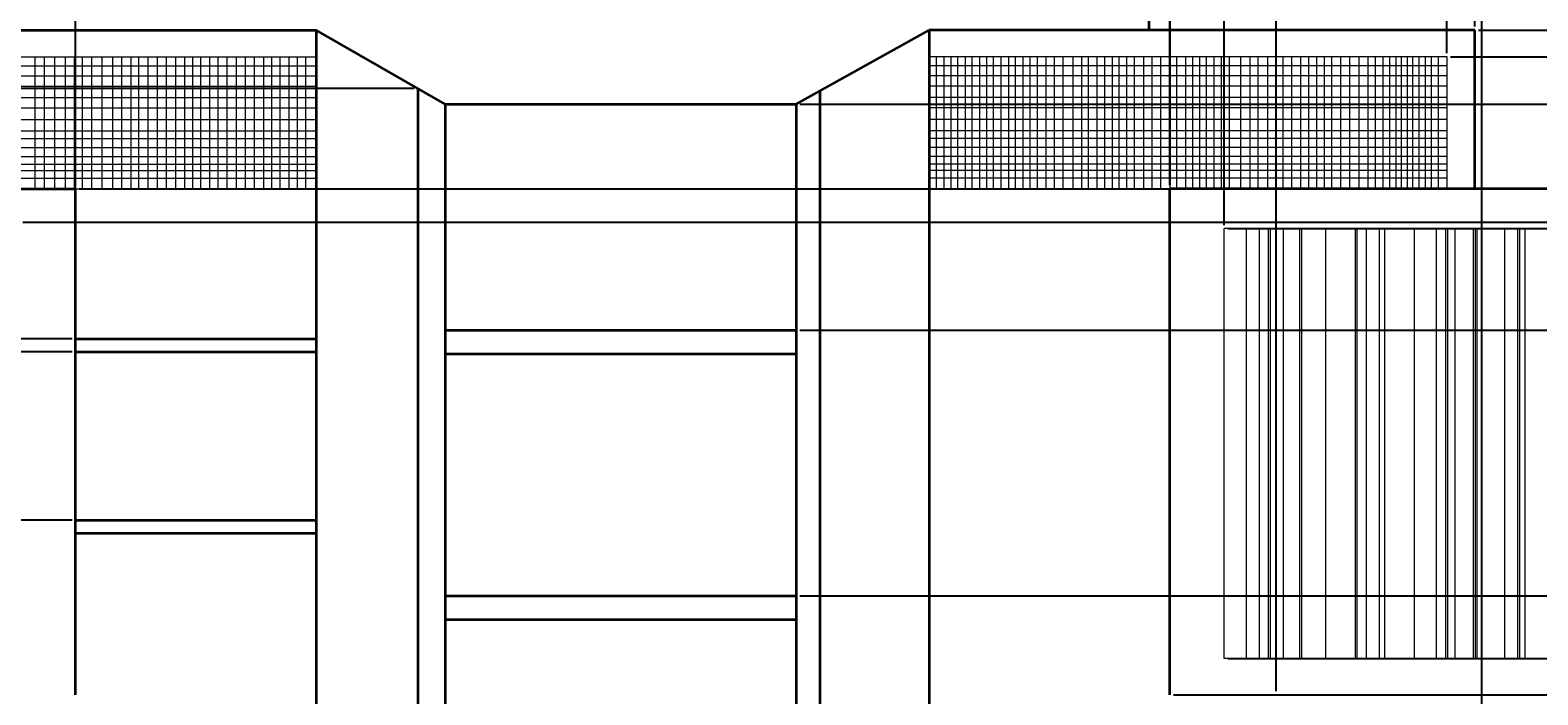
# Model space of a CAD drawing. Units: inches. Extents: x -10 to 130, y -32 to 34.
# Tile 16 of 22: x 49 to 75, y 6 to 18. Entities that reach past the tile are written whole.
import ezdxf

# ---------------------------------------------------------------- set-up
doc = ezdxf.new("R2010")
doc.units = ezdxf.units.IN
doc.header["$MEASUREMENT"] = 0
for name, color, linetype, lineweight in [('A-ANNO-DIMS', 2, 'Continuous', 18), ('A-ELEV', 7, 'Continuous', 35), ('A-GLAZ', 4, 'Continuous', 18)]:
    doc.layers.add(name, color=color, linetype=linetype, lineweight=lineweight)
doc.styles.get("Standard").update_dxf_attribs({"font": 'arial.ttf'})
doc.dimstyles.get("Standard").update_dxf_attribs({"dimtxt": 0.18, "dimasz": 0.18, "dimexe": 0.18, "dimexo": 0.0625, "dimgap": 0.09, "dimtad": 0, "dimtih": 1, "dimtoh": 1, "dimdec": 4, "dimzin": 0, "dimdsep": 46, "dimtxsty": 'Standard', "dimcen": 0.09, "dimadec": 0, "dimazin": 0, "dimtfac": 1, "dimtdec": 4, "dimtofl": 0, "dimtmove": 0, "dimatfit": 3, "dimfxl": 1, "dimtolj": 1, "dimtzin": 0, "dimarcsym": 0})

# ---------------------------------------------------------------- blocks, each defined once
blk = doc.blocks.new('*D2')
at = {"layer": 'A-ANNO-DIMS', "color": 0, "lineweight": -2, "transparency": 16777216}
for p, q in [((68.738, 27.199), (129.508, 27.199)), ((129.328, 27.019), (129.328, 3.074)), ((129.328, -21.234), (129.328, 2.71)), ((107.996, -21.414), (129.508, -21.414))]:
    blk.add_line(p, q, dxfattribs=at)
at = {"layer": 'A-ANNO-DIMS', "color": 0, "transparency": 16777216}
for points in [[(129.298, 27.019), (129.358, 27.019), (129.328, 27.199)], [(129.298, -21.234), (129.358, -21.234), (129.328, -21.414)]]:
    blk.add_solid(points, dxfattribs=at)
at = {"layer": 'Defpoints', "color": 0, "transparency": 16777216}
for p in [(68.676, 27.199), (129.328, 27.199), (107.933, -21.414)]:
    blk.add_point(p, dxfattribs=at)
at = {"layer": 'A-ANNO-DIMS', "color": 0, "transparency": 16777216, "insert": (129.328, 2.892), "char_height": 0.18, "attachment_point": 5}
blk.add_mtext('\\A1;48.61', dxfattribs=at)
blk = doc.blocks.new('*D7')
at = {"layer": 'A-ANNO-DIMS', "color": 0, "lineweight": -2, "transparency": 16777216}
for p, q in [((42.614, 6.07), (42.614, 33.879)), ((42.794, 33.699), (45.888, 33.699)), ((49.766, 33.699), (46.672, 33.699)), ((49.946, 6.07), (49.946, 33.879))]:
    blk.add_line(p, q, dxfattribs=at)
at = {"layer": 'A-ANNO-DIMS', "color": 0, "transparency": 16777216}
for points in [[(42.794, 33.729), (42.794, 33.669), (42.614, 33.699)], [(49.766, 33.729), (49.766, 33.669), (49.946, 33.699)]]:
    blk.add_solid(points, dxfattribs=at)
at = {"layer": 'Defpoints', "color": 0, "transparency": 16777216}
for p in [(49.946, 33.699), (42.614, 6.007), (49.946, 6.007)]:
    blk.add_point(p, dxfattribs=at)
at = {"layer": 'A-ANNO-DIMS', "color": 0, "transparency": 16777216, "insert": (46.28, 33.699), "char_height": 0.18, "attachment_point": 5}
blk.add_mtext('\\A1;7.332', dxfattribs=at)
blk = doc.blocks.new('*D8')
at = {"layer": 'A-ANNO-DIMS', "color": 0, "lineweight": -2, "transparency": 16777216}
for p, q in [((68.676, 17.67), (68.676, 33.879)), ((68.856, 33.699), (69.393, 33.699)), ((70.718, 33.699), (70.181, 33.699)), ((70.898, 6.07), (70.898, 33.879))]:
    blk.add_line(p, q, dxfattribs=at)
at = {"layer": 'A-ANNO-DIMS', "color": 0, "transparency": 16777216}
for points in [[(68.856, 33.729), (68.856, 33.669), (68.676, 33.699)], [(70.718, 33.729), (70.718, 33.669), (70.898, 33.699)]]:
    blk.add_solid(points, dxfattribs=at)
at = {"layer": 'Defpoints', "color": 0, "transparency": 16777216}
for p in [(70.898, 33.699), (68.676, 17.607), (70.898, 6.007)]:
    blk.add_point(p, dxfattribs=at)
at = {"layer": 'A-ANNO-DIMS', "color": 0, "transparency": 16777216, "insert": (69.787, 33.699), "char_height": 0.18, "attachment_point": 5}
blk.add_mtext('\\A1;2.222', dxfattribs=at)
blk = doc.blocks.new('*D9')
at = {"layer": 'A-ANNO-DIMS', "color": 0, "lineweight": -2, "transparency": 16777216}
for p, q in [((70.898, 6.07), (70.898, 33.879)), ((71.078, 33.699), (75.697, 33.699)), ((81.225, 33.699), (76.607, 33.699)), ((81.405, 6.07), (81.405, 33.879))]:
    blk.add_line(p, q, dxfattribs=at)
at = {"layer": 'A-ANNO-DIMS', "color": 0, "transparency": 16777216}
for points in [[(71.078, 33.729), (71.078, 33.669), (70.898, 33.699)], [(81.225, 33.729), (81.225, 33.669), (81.405, 33.699)]]:
    blk.add_solid(points, dxfattribs=at)
at = {"layer": 'Defpoints', "color": 0, "transparency": 16777216}
for p in [(81.405, 33.699), (70.898, 6.007), (81.405, 6.007)]:
    blk.add_point(p, dxfattribs=at)
at = {"layer": 'A-ANNO-DIMS', "color": 0, "transparency": 16777216, "insert": (76.152, 33.699), "char_height": 0.18, "attachment_point": 5}
blk.add_mtext('\\A1;10.507', dxfattribs=at)
blk = doc.blocks.new('*D28')
at = {"layer": 'A-ANNO-DIMS', "color": 0, "lineweight": -2, "transparency": 16777216}
for p, q in [((21.715, 14.903), (21.715, 33.879)), ((21.895, 33.699), (35.436, 33.699)), ((49.766, 33.699), (36.226, 33.699)), ((49.946, 14.903), (49.946, 33.879))]:
    blk.add_line(p, q, dxfattribs=at)
at = {"layer": 'A-ANNO-DIMS', "color": 0, "transparency": 16777216}
for points in [[(21.895, 33.729), (21.895, 33.669), (21.715, 33.699)], [(49.766, 33.729), (49.766, 33.669), (49.946, 33.699)]]:
    blk.add_solid(points, dxfattribs=at)
at = {"layer": 'Defpoints', "color": 0, "transparency": 16777216}
for p in [(49.946, 33.699), (21.715, 14.841), (49.946, 14.841)]:
    blk.add_point(p, dxfattribs=at)
at = {"layer": 'A-ANNO-DIMS', "color": 0, "transparency": 16777216, "insert": (35.831, 33.699), "char_height": 0.18, "attachment_point": 5}
blk.add_mtext('\\A1;28.23', dxfattribs=at)
blk = doc.blocks.new('*D29')
at = {"layer": 'A-ANNO-DIMS', "color": 0, "lineweight": -2, "transparency": 16777216}
for p, q in [((69.045, 14.903), (69.045, 33.879)), ((69.225, 33.699), (82.743, 33.699)), ((97.053, 33.699), (83.534, 33.699)), ((97.233, 14.903), (97.233, 33.879))]:
    blk.add_line(p, q, dxfattribs=at)
at = {"layer": 'A-ANNO-DIMS', "color": 0, "transparency": 16777216}
for points in [[(69.225, 33.729), (69.225, 33.669), (69.045, 33.699)], [(97.053, 33.729), (97.053, 33.669), (97.233, 33.699)]]:
    blk.add_solid(points, dxfattribs=at)
at = {"layer": 'Defpoints', "color": 0, "transparency": 16777216}
for p in [(97.233, 33.699), (69.045, 14.841), (97.233, 14.841)]:
    blk.add_point(p, dxfattribs=at)
at = {"layer": 'A-ANNO-DIMS', "color": 0, "transparency": 16777216, "insert": (83.139, 33.699), "char_height": 0.18, "attachment_point": 5}
blk.add_mtext('\\A1;28.19', dxfattribs=at)
blk = doc.blocks.new('*D34')
at = {"layer": 'A-ANNO-DIMS', "color": 0, "lineweight": -2, "transparency": 16777216}
for p, q in [((13.34, 6.007), (-9.564, 6.007)), ((-9.384, 5.827), (-9.384, 3.941)), ((-9.384, 1.691), (-9.384, 3.577)), ((70.835, 1.511), (-9.564, 1.511))]:
    blk.add_line(p, q, dxfattribs=at)
at = {"layer": 'A-ANNO-DIMS', "color": 0, "transparency": 16777216}
for points in [[(-9.414, 5.827), (-9.354, 5.827), (-9.384, 6.007)], [(-9.414, 1.691), (-9.354, 1.691), (-9.384, 1.511)]]:
    blk.add_solid(points, dxfattribs=at)
at = {"layer": 'Defpoints', "color": 0, "transparency": 16777216}
for p in [(-9.384, 6.007), (13.402, 6.007), (70.898, 1.511)]:
    blk.add_point(p, dxfattribs=at)
at = {"layer": 'A-ANNO-DIMS', "color": 0, "transparency": 16777216, "insert": (-9.384, 3.759), "char_height": 0.18, "attachment_point": 5}
blk.add_mtext('\\A1;4.497', dxfattribs=at)
blk = doc.blocks.new('*D48')
at = {"layer": 'A-ANNO-DIMS', "color": 0, "lineweight": -2, "transparency": 16777216}
for p, q in [((44.76, -13.293), (44.76, 33.879)), ((44.94, 33.699), (59.231, 33.699)), ((74.312, 33.699), (60.021, 33.699)), ((74.492, -13.293), (74.492, 33.879))]:
    blk.add_line(p, q, dxfattribs=at)
at = {"layer": 'A-ANNO-DIMS', "color": 0, "transparency": 16777216}
for points in [[(44.94, 33.729), (44.94, 33.669), (44.76, 33.699)], [(74.312, 33.729), (74.312, 33.669), (74.492, 33.699)]]:
    blk.add_solid(points, dxfattribs=at)
at = {"layer": 'Defpoints', "color": 0, "transparency": 16777216}
for p in [(74.492, 33.699), (44.76, -13.356), (74.492, -13.356)]:
    blk.add_point(p, dxfattribs=at)
at = {"layer": 'A-ANNO-DIMS', "color": 0, "transparency": 16777216, "insert": (59.626, 33.699), "char_height": 0.18, "attachment_point": 5}
blk.add_mtext('\\A1;29.73', dxfattribs=at)
blk = doc.blocks.new('*D60')
at = {"layer": 'A-ANNO-DIMS', "color": 0, "lineweight": -2, "transparency": 16777216}
for p, q in [((74.492, -13.293), (74.492, 33.879)), ((74.672, 33.699), (78.041, 33.699)), ((82.197, 33.699), (78.828, 33.699)), ((82.377, -15.202), (82.377, 33.879))]:
    blk.add_line(p, q, dxfattribs=at)
at = {"layer": 'A-ANNO-DIMS', "color": 0, "transparency": 16777216}
for points in [[(74.672, 33.729), (74.672, 33.669), (74.492, 33.699)], [(82.197, 33.729), (82.197, 33.669), (82.377, 33.699)]]:
    blk.add_solid(points, dxfattribs=at)
at = {"layer": 'Defpoints', "color": 0, "transparency": 16777216}
for p in [(82.377, 33.699), (74.492, -13.356), (82.377, -15.264)]:
    blk.add_point(p, dxfattribs=at)
at = {"layer": 'A-ANNO-DIMS', "color": 0, "transparency": 16777216, "insert": (78.435, 33.699), "char_height": 0.18, "attachment_point": 5}
blk.add_mtext('\\A1;7.885', dxfattribs=at)
blk = doc.blocks.new('*D72')
at = {"layer": 'A-ANNO-DIMS', "color": 0, "lineweight": -2, "transparency": 16777216}
for p, q in [((55.918, 16.529), (55.918, -28.129)), ((62.934, 16.482), (62.934, -28.129)), ((56.098, -27.949), (59.033, -27.949)), ((62.754, -27.949), (59.819, -27.949))]:
    blk.add_line(p, q, dxfattribs=at)
at = {"layer": 'A-ANNO-DIMS', "color": 0, "transparency": 16777216}
for points in [[(56.098, -27.919), (56.098, -27.979), (55.918, -27.949)], [(62.754, -27.919), (62.754, -27.979), (62.934, -27.949)]]:
    blk.add_solid(points, dxfattribs=at)
at = {"layer": 'Defpoints', "color": 0, "transparency": 16777216}
for p in [(55.918, 16.591), (62.934, 16.545), (62.934, -27.949)]:
    blk.add_point(p, dxfattribs=at)
at = {"layer": 'A-ANNO-DIMS', "color": 0, "transparency": 16777216, "insert": (59.426, -27.949), "char_height": 0.18, "attachment_point": 5}
blk.add_mtext('\\A1;7.016', dxfattribs=at)
blk = doc.blocks.new('*D73')
at = {"layer": 'A-ANNO-DIMS', "color": 0, "lineweight": -2, "transparency": 16777216}
for p, q in [((56.395, 16.255), (56.395, -28.129)), ((62.526, 16.255), (62.526, -28.129)), ((56.575, -27.949), (59.083, -27.949)), ((62.346, -27.949), (59.837, -27.949))]:
    blk.add_line(p, q, dxfattribs=at)
at = {"layer": 'A-ANNO-DIMS', "color": 0, "transparency": 16777216}
for points in [[(56.575, -27.919), (56.575, -27.979), (56.395, -27.949)], [(62.346, -27.919), (62.346, -27.979), (62.526, -27.949)]]:
    blk.add_solid(points, dxfattribs=at)
at = {"layer": 'Defpoints', "color": 0, "transparency": 16777216}
for p in [(56.395, 16.317), (62.526, 16.317), (62.526, -27.949)]:
    blk.add_point(p, dxfattribs=at)
at = {"layer": 'A-ANNO-DIMS', "color": 0, "transparency": 16777216, "insert": (59.46, -27.949), "char_height": 0.18, "attachment_point": 5}
blk.add_mtext('\\A1;6.131', dxfattribs=at)
blk = doc.blocks.new('*D74')
at = {"layer": 'A-ANNO-DIMS', "color": 0, "lineweight": -2, "transparency": 16777216}
for p, q in [((54.085, 17.607), (-9.564, 17.607)), ((-9.384, 17.427), (-9.384, 17.281)), ((-9.384, 16.771), (-9.384, 16.917)), ((55.856, 16.591), (-9.564, 16.591))]:
    blk.add_line(p, q, dxfattribs=at)
at = {"layer": 'A-ANNO-DIMS', "color": 0, "transparency": 16777216}
for points in [[(-9.414, 17.427), (-9.354, 17.427), (-9.384, 17.607)], [(-9.414, 16.771), (-9.354, 16.771), (-9.384, 16.591)]]:
    blk.add_solid(points, dxfattribs=at)
at = {"layer": 'Defpoints', "color": 0, "transparency": 16777216}
for p in [(54.147, 17.607), (-9.384, 16.591), (55.918, 16.591)]:
    blk.add_point(p, dxfattribs=at)
at = {"layer": 'A-ANNO-DIMS', "color": 0, "transparency": 16777216, "insert": (-9.384, 17.099), "char_height": 0.18, "attachment_point": 5}
blk.add_mtext('\\A1;1.02', dxfattribs=at)
blk = doc.blocks.new('*D79')
at = {"layer": 'A-ANNO-DIMS', "color": 0, "lineweight": -2, "transparency": 16777216}
for p, q in [((62.588, 7.736), (129.508, 7.736)), ((129.328, 7.556), (129.328, 5.559)), ((129.328, 3.198), (129.328, 5.195)), ((62.588, 3.018), (129.508, 3.018))]:
    blk.add_line(p, q, dxfattribs=at)
at = {"layer": 'A-ANNO-DIMS', "color": 0, "transparency": 16777216}
for points in [[(129.298, 7.556), (129.358, 7.556), (129.328, 7.736)], [(129.298, 3.198), (129.358, 3.198), (129.328, 3.018)]]:
    blk.add_solid(points, dxfattribs=at)
at = {"layer": 'Defpoints', "color": 0, "transparency": 16777216}
for p in [(62.526, 7.736), (129.328, 7.736), (62.526, 3.018)]:
    blk.add_point(p, dxfattribs=at)
at = {"layer": 'A-ANNO-DIMS', "color": 0, "transparency": 16777216, "insert": (129.328, 5.377), "char_height": 0.18, "attachment_point": 5}
blk.add_mtext('\\A1;4.718', dxfattribs=at)
blk = doc.blocks.new('*D80')
at = {"layer": 'A-ANNO-DIMS', "color": 0, "lineweight": -2, "transparency": 16777216}
for p, q in [((62.588, 12.373), (129.508, 12.373)), ((129.328, 12.193), (129.328, 10.237)), ((129.328, 7.916), (129.328, 9.873)), ((62.588, 7.736), (129.508, 7.736))]:
    blk.add_line(p, q, dxfattribs=at)
at = {"layer": 'A-ANNO-DIMS', "color": 0, "transparency": 16777216}
for points in [[(129.298, 12.193), (129.358, 12.193), (129.328, 12.373)], [(129.298, 7.916), (129.358, 7.916), (129.328, 7.736)]]:
    blk.add_solid(points, dxfattribs=at)
at = {"layer": 'Defpoints', "color": 0, "transparency": 16777216}
for p in [(62.526, 12.373), (129.328, 12.373), (62.526, 7.736)]:
    blk.add_point(p, dxfattribs=at)
at = {"layer": 'A-ANNO-DIMS', "color": 0, "transparency": 16777216, "insert": (129.328, 10.055), "char_height": 0.18, "attachment_point": 5}
blk.add_mtext('\\A1;4.64', dxfattribs=at)
blk = doc.blocks.new('*D81')
at = {"layer": 'A-ANNO-DIMS', "color": 0, "lineweight": -2, "transparency": 16777216}
for p, q in [((62.588, 16.317), (129.508, 16.317)), ((129.328, 16.137), (129.328, 14.527)), ((129.328, 12.553), (129.328, 14.163)), ((62.588, 12.373), (129.508, 12.373))]:
    blk.add_line(p, q, dxfattribs=at)
at = {"layer": 'A-ANNO-DIMS', "color": 0, "transparency": 16777216}
for points in [[(129.298, 16.137), (129.358, 16.137), (129.328, 16.317)], [(129.298, 12.553), (129.358, 12.553), (129.328, 12.373)]]:
    blk.add_solid(points, dxfattribs=at)
at = {"layer": 'Defpoints', "color": 0, "transparency": 16777216}
for p in [(62.526, 16.317), (129.328, 16.317), (62.526, 12.373)]:
    blk.add_point(p, dxfattribs=at)
at = {"layer": 'A-ANNO-DIMS', "color": 0, "transparency": 16777216, "insert": (129.328, 14.345), "char_height": 0.18, "attachment_point": 5}
blk.add_mtext('\\A1;3.94', dxfattribs=at)
blk = doc.blocks.new('*D87')
at = {"layer": 'A-ANNO-DIMS', "color": 0, "lineweight": -2, "transparency": 16777216}
for p, q in [((49.884, 14.841), (-9.564, 14.841)), ((-9.384, 14.661), (-9.384, 13.713)), ((-9.384, 12.402), (-9.384, 13.35)), ((49.884, 12.222), (-9.564, 12.222))]:
    blk.add_line(p, q, dxfattribs=at)
at = {"layer": 'A-ANNO-DIMS', "color": 0, "transparency": 16777216}
for points in [[(-9.414, 14.661), (-9.354, 14.661), (-9.384, 14.841)], [(-9.414, 12.402), (-9.354, 12.402), (-9.384, 12.222)]]:
    blk.add_solid(points, dxfattribs=at)
at = {"layer": 'Defpoints', "color": 0, "transparency": 16777216}
for p in [(49.946, 14.841), (-9.384, 12.222), (49.946, 12.222)]:
    blk.add_point(p, dxfattribs=at)
at = {"layer": 'A-ANNO-DIMS', "color": 0, "transparency": 16777216, "insert": (-9.384, 13.532), "char_height": 0.18, "attachment_point": 5}
blk.add_mtext('\\A1;2.619', dxfattribs=at)
blk = doc.blocks.new('*D88')
at = {"layer": 'A-ANNO-DIMS', "color": 0, "lineweight": -2, "transparency": 16777216}
for p, q in [((49.884, 12.222), (-9.564, 12.222)), ((-9.384, 12.042), (-9.384, 10.822)), ((-9.384, 9.238), (-9.384, 10.458)), ((49.884, 9.058), (-9.564, 9.058))]:
    blk.add_line(p, q, dxfattribs=at)
at = {"layer": 'A-ANNO-DIMS', "color": 0, "transparency": 16777216}
for points in [[(-9.414, 12.042), (-9.354, 12.042), (-9.384, 12.222)], [(-9.414, 9.238), (-9.354, 9.238), (-9.384, 9.058)]]:
    blk.add_solid(points, dxfattribs=at)
at = {"layer": 'Defpoints', "color": 0, "transparency": 16777216}
for p in [(49.946, 12.222), (-9.384, 9.058), (49.946, 9.058)]:
    blk.add_point(p, dxfattribs=at)
at = {"layer": 'A-ANNO-DIMS', "color": 0, "transparency": 16777216, "insert": (-9.384, 10.64), "char_height": 0.18, "attachment_point": 5}
blk.add_mtext('\\A1;3.164', dxfattribs=at)
blk = doc.blocks.new('*D89')
at = {"layer": 'A-ANNO-DIMS', "color": 0, "lineweight": -2, "transparency": 16777216}
for p, q in [((49.884, 9.058), (-9.564, 9.058)), ((-9.384, 8.878), (-9.384, 7.612)), ((-9.384, 5.982), (-9.384, 7.248)), ((49.884, 5.802), (-9.564, 5.802))]:
    blk.add_line(p, q, dxfattribs=at)
at = {"layer": 'A-ANNO-DIMS', "color": 0, "transparency": 16777216}
for points in [[(-9.414, 8.878), (-9.354, 8.878), (-9.384, 9.058)], [(-9.414, 5.982), (-9.354, 5.982), (-9.384, 5.802)]]:
    blk.add_solid(points, dxfattribs=at)
at = {"layer": 'Defpoints', "color": 0, "transparency": 16777216}
for p in [(49.946, 9.058), (-9.384, 5.802), (49.946, 5.802)]:
    blk.add_point(p, dxfattribs=at)
at = {"layer": 'A-ANNO-DIMS', "color": 0, "transparency": 16777216, "insert": (-9.384, 7.43), "char_height": 0.18, "attachment_point": 5}
blk.add_mtext('\\A1;3.256', dxfattribs=at)
blk = doc.blocks.new('*D95')
at = {"layer": 'A-ANNO-DIMS', "color": 0, "lineweight": -2, "transparency": 16777216}
for p, q in [((-9.384, 12.402), (-9.384, 12.582)), ((49.884, 12.222), (-9.564, 12.222)), ((49.884, 11.995), (-9.564, 11.995)), ((-9.384, 11.635), (-9.564, 11.635)), ((-9.384, 11.815), (-9.384, 11.635))]:
    blk.add_line(p, q, dxfattribs=at)
at = {"layer": 'A-ANNO-DIMS', "color": 0, "transparency": 16777216}
for points in [[(-9.414, 12.402), (-9.354, 12.402), (-9.384, 12.222)], [(-9.414, 11.815), (-9.354, 11.815), (-9.384, 11.995)]]:
    blk.add_solid(points, dxfattribs=at)
at = {"layer": 'Defpoints', "color": 0, "transparency": 16777216}
for p in [(49.946, 12.222), (-9.384, 11.995), (49.946, 11.995)]:
    blk.add_point(p, dxfattribs=at)
at = {"layer": 'A-ANNO-DIMS', "color": 0, "transparency": 16777216, "insert": (-9.957, 11.635), "char_height": 0.18, "attachment_point": 5}
blk.add_mtext('\\A1;0.227', dxfattribs=at)
blk = doc.blocks.new('*D107')
at = {"layer": 'A-ANNO-DIMS', "color": 0, "lineweight": -2, "transparency": 16777216}
for p, q in [((48.783, 33.699), (48.603, 33.699)), ((48.963, 14.318), (48.963, 33.879)), ((49.946, 14.903), (49.946, 33.879)), ((50.126, 33.699), (50.306, 33.699))]:
    blk.add_line(p, q, dxfattribs=at)
at = {"layer": 'A-ANNO-DIMS', "color": 0, "transparency": 16777216}
for points in [[(48.783, 33.729), (48.783, 33.669), (48.963, 33.699)], [(50.126, 33.729), (50.126, 33.669), (49.946, 33.699)]]:
    blk.add_solid(points, dxfattribs=at)
at = {"layer": 'Defpoints', "color": 0, "transparency": 16777216}
for p in [(49.946, 33.699), (49.946, 14.841), (48.963, 14.256)]:
    blk.add_point(p, dxfattribs=at)
at = {"layer": 'A-ANNO-DIMS', "color": 0, "transparency": 16777216, "insert": (49.455, 33.699), "char_height": 0.18, "attachment_point": 5}
blk.add_mtext('\\A1;0.983', dxfattribs=at)
blk = doc.blocks.new('*D108')
at = {"layer": 'A-ANNO-DIMS', "color": 0, "lineweight": -2, "transparency": 16777216}
for p, q in [((129.328, 14.841), (129.328, 15.021)), ((129.328, 15.021), (129.508, 15.021)), ((50.009, 14.841), (129.508, 14.841)), ((129.328, 14.436), (129.328, 14.661)), ((49.025, 14.256), (129.508, 14.256))]:
    blk.add_line(p, q, dxfattribs=at)
at = {"layer": 'A-ANNO-DIMS', "color": 0, "transparency": 16777216}
for points in [[(129.298, 14.661), (129.358, 14.661), (129.328, 14.841)], [(129.298, 14.436), (129.358, 14.436), (129.328, 14.256)]]:
    blk.add_solid(points, dxfattribs=at)
at = {"layer": 'Defpoints', "color": 0, "transparency": 16777216}
for p in [(49.946, 14.841), (129.328, 14.841), (48.963, 14.256)]:
    blk.add_point(p, dxfattribs=at)
at = {"layer": 'A-ANNO-DIMS', "color": 0, "transparency": 16777216, "insert": (129.902, 15.021), "char_height": 0.18, "attachment_point": 5}
blk.add_mtext('\\A1;0.585', dxfattribs=at)
blk = doc.blocks.new('*D136')
at = {"layer": 'A-ANNO-DIMS', "color": 0, "lineweight": -2, "transparency": 16777216}
for p, q in [((68.87, 33.699), (68.69, 33.699)), ((69.05, 14.903), (69.05, 33.879)), ((69.995, 14.206), (69.995, 33.879)), ((70.175, 33.699), (70.355, 33.699))]:
    blk.add_line(p, q, dxfattribs=at)
at = {"layer": 'A-ANNO-DIMS', "color": 0, "transparency": 16777216}
for points in [[(68.87, 33.729), (68.87, 33.669), (69.05, 33.699)], [(70.175, 33.729), (70.175, 33.669), (69.995, 33.699)]]:
    blk.add_solid(points, dxfattribs=at)
at = {"layer": 'Defpoints', "color": 0, "transparency": 16777216}
for p in [(69.995, 33.699), (69.05, 14.841), (69.995, 14.144)]:
    blk.add_point(p, dxfattribs=at)
at = {"layer": 'A-ANNO-DIMS', "color": 0, "transparency": 16777216, "insert": (69.522, 33.699), "char_height": 0.18, "attachment_point": 5}
blk.add_mtext('\\A1;0.945', dxfattribs=at)
blk = doc.blocks.new('*D137')
at = {"layer": 'A-ANNO-DIMS', "color": 0, "lineweight": -2, "transparency": 16777216}
for p, q in [((69.995, 14.206), (69.995, 33.879)), ((70.175, 33.699), (82.678, 33.699)), ((96.113, 33.699), (83.609, 33.699)), ((96.293, 14.206), (96.293, 33.879))]:
    blk.add_line(p, q, dxfattribs=at)
at = {"layer": 'A-ANNO-DIMS', "color": 0, "transparency": 16777216}
for points in [[(70.175, 33.729), (70.175, 33.669), (69.995, 33.699)], [(96.113, 33.729), (96.113, 33.669), (96.293, 33.699)]]:
    blk.add_solid(points, dxfattribs=at)
at = {"layer": 'Defpoints', "color": 0, "transparency": 16777216}
for p in [(96.293, 33.699), (69.995, 14.144), (96.293, 14.144)]:
    blk.add_point(p, dxfattribs=at)
at = {"layer": 'A-ANNO-DIMS', "color": 0, "transparency": 16777216, "insert": (83.144, 33.699), "char_height": 0.18, "attachment_point": 5}
blk.add_mtext('\\A1;26.298', dxfattribs=at)
blk = doc.blocks.new('*D138')
at = {"layer": 'A-ANNO-DIMS', "color": 0, "lineweight": -2, "transparency": 16777216}
for p, q in [((129.328, 14.841), (129.328, 15.021)), ((129.328, 15.021), (129.508, 15.021)), ((69.112, 14.841), (129.508, 14.841)), ((129.328, 14.324), (129.328, 14.661)), ((70.057, 14.144), (129.508, 14.144))]:
    blk.add_line(p, q, dxfattribs=at)
at = {"layer": 'A-ANNO-DIMS', "color": 0, "transparency": 16777216}
for points in [[(129.298, 14.661), (129.358, 14.661), (129.328, 14.841)], [(129.298, 14.324), (129.358, 14.324), (129.328, 14.144)]]:
    blk.add_solid(points, dxfattribs=at)
at = {"layer": 'Defpoints', "color": 0, "transparency": 16777216}
for p in [(69.05, 14.841), (129.328, 14.841), (69.995, 14.144)]:
    blk.add_point(p, dxfattribs=at)
at = {"layer": 'A-ANNO-DIMS', "color": 0, "transparency": 16777216, "insert": (129.901, 15.021), "char_height": 0.18, "attachment_point": 5}
blk.add_mtext('\\A1;0.697', dxfattribs=at)
blk = doc.blocks.new('*D139')
at = {"layer": 'A-ANNO-DIMS', "color": 0, "lineweight": -2, "transparency": 16777216}
for p, q in [((70.057, 6.643), (129.508, 6.643)), ((129.328, 6.463), (129.328, 6.187)), ((69.108, 6.007), (129.508, 6.007)), ((129.328, 5.827), (129.148, 5.827)), ((129.328, 6.007), (129.328, 5.827))]:
    blk.add_line(p, q, dxfattribs=at)
at = {"layer": 'A-ANNO-DIMS', "color": 0, "transparency": 16777216}
for points in [[(129.298, 6.463), (129.358, 6.463), (129.328, 6.643)], [(129.298, 6.187), (129.358, 6.187), (129.328, 6.007)]]:
    blk.add_solid(points, dxfattribs=at)
at = {"layer": 'Defpoints', "color": 0, "transparency": 16777216}
for p in [(69.995, 6.643), (69.045, 6.007), (129.328, 6.007)]:
    blk.add_point(p, dxfattribs=at)
at = {"layer": 'A-ANNO-DIMS', "color": 0, "transparency": 16777216, "insert": (128.754, 5.827), "char_height": 0.18, "attachment_point": 5}
blk.add_mtext('\\A1;0.636', dxfattribs=at)
blk = doc.blocks.new('*D149')
at = {"layer": 'A-ANNO-DIMS', "color": 0, "lineweight": -2, "transparency": 16777216}
for p, q in [((73.702, 33.699), (73.522, 33.699)), ((73.882, 17.205), (73.882, 33.879)), ((74.37, 17.67), (74.37, 33.879)), ((74.55, 33.699), (74.73, 33.699))]:
    blk.add_line(p, q, dxfattribs=at)
at = {"layer": 'A-ANNO-DIMS', "color": 0, "transparency": 16777216}
for points in [[(73.702, 33.729), (73.702, 33.669), (73.882, 33.699)], [(74.55, 33.729), (74.55, 33.669), (74.37, 33.699)]]:
    blk.add_solid(points, dxfattribs=at)
at = {"layer": 'Defpoints', "color": 0, "transparency": 16777216}
for p in [(74.37, 33.699), (74.37, 17.607), (73.882, 17.143)]:
    blk.add_point(p, dxfattribs=at)
at = {"layer": 'A-ANNO-DIMS', "color": 0, "transparency": 16777216, "insert": (75.123, 33.699), "char_height": 0.18, "attachment_point": 5}
blk.add_mtext('\\A1;0.487', dxfattribs=at)
blk = doc.blocks.new('*D150')
at = {"layer": 'A-ANNO-DIMS', "color": 0, "lineweight": -2, "transparency": 16777216}
for p, q in [((129.327673, 17.787359), (129.327673, 17.967359)), ((74.432221, 17.607359), (129.507673, 17.607359)), ((73.944831, 17.142679), (129.507673, 17.142679)), ((129.327673, 16.962679), (129.327673, 16.782679))]:
    blk.add_line(p, q, dxfattribs=at)
at = {"layer": 'A-ANNO-DIMS', "color": 0, "transparency": 16777216}
for points in [[(129.297673, 17.787359), (129.357673, 17.787359), (129.327673, 17.607359)], [(129.297673, 16.962679), (129.357673, 16.962679), (129.327673, 17.142679)]]:
    blk.add_solid(points, dxfattribs=at)
at = {"layer": 'Defpoints', "color": 0, "transparency": 16777216}
for p in [(74.369721, 17.607359), (129.327673, 17.607359), (73.882331, 17.142679)]:
    blk.add_point(p, dxfattribs=at)
at = {"layer": 'A-ANNO-DIMS', "color": 0, "transparency": 16777216, "insert": (129.327673, 17.375019), "char_height": 0.18, "attachment_point": 5}
blk.add_mtext('\\A1;0.465', dxfattribs=at)

msp = doc.modelspace()

# ---------------------------------------------------------------- linework, layer by layer
at = {"layer": 'A-ELEV'}
for p, q in [((68.6759, 27.1987), (68.6759, 17.6074)), ((44.6217, 17.6074), (54.1471, 17.6074)), ((54.1471, 17.6074), (54.1471, -13.3558)), ((56.395, 16.3174), (54.1471, 17.6074)), ((62.5256, 16.3174), (64.8443, 17.6074)), ((74.3697, 17.6074), (64.8443, 17.6074)), ((64.8443, 17.6074), (64.8443, -13.3558)), ((74.3697, 14.8409), (74.3697, 17.6074)), ((55.9182, 16.5911), (55.9182, -13.3558)), ((56.395, 16.3174), (56.395, -13.3558)), ((56.395, 16.3174), (62.5256, 16.3174)), ((62.5256, 16.3174), (62.5256, -13.3558)), ((62.9343, 16.5448), (62.9343, -13.3558)), ((21.7155, 14.8409), (49.9462, 14.8409)), ((49.9462, 6.0074), (49.9462, 14.8409)), ((97.276, 14.8409), (69.0452, 14.8409)), ((69.0452, 6.0074), (69.0452, 14.8409)), ((56.395, 12.3729), (62.5256, 12.3729)), ((49.9462, 12.2222), (54.1471, 12.2222)), ((49.9462, 11.9951), (54.1471, 11.9951)), ((56.395, 11.9577), (62.5256, 11.9577)), ((49.9462, 9.058), (54.1471, 9.058)), ((49.9462, 8.8309), (54.1471, 8.8309)), ((56.395, 7.7364), (62.5256, 7.7364)), ((56.395, 7.3212), (62.5256, 7.3212))]:
    msp.add_line(p, q, dxfattribs=at)
at = {"layer": 'A-GLAZ'}
for p, q in [((45.1026, 17.1427), (54.1471, 17.1427)), ((49.2418, 14.8409), (49.2418, 17.1427)), ((49.4023, 14.8409), (49.4023, 17.1427)), ((49.5856, 14.8409), (49.5856, 17.1427)), ((49.769, 14.8409), (49.769, 17.1427)), ((49.9294, 14.8409), (49.9294, 17.1427)), ((50.0669, 14.8409), (50.0669, 17.1427)), ((50.2274, 14.8409), (50.2274, 17.1427)), ((50.4107, 14.8409), (50.4107, 17.1427)), ((50.5941, 14.8409), (50.5941, 17.1427)), ((50.7545, 14.8409), (50.7545, 17.1427)), ((50.915, 14.8409), (50.915, 17.1427)), ((51.0525, 14.8409), (51.0525, 17.1427)), ((51.2129, 14.8409), (51.2129, 17.1427)), ((51.3733, 14.8409), (51.3733, 17.1427)), ((51.5338, 14.8409), (51.5338, 17.1427)), ((51.6942, 14.8409), (51.6942, 17.1427)), ((51.8546, 14.8409), (51.8546, 17.1427)), ((51.9922, 14.8409), (51.9922, 17.1427)), ((52.1328, 14.8409), (52.1328, 17.1427)), ((52.2915, 14.8409), (52.2915, 17.1427)), ((52.4357, 14.8409), (52.4357, 17.1427)), ((52.5944, 14.8409), (52.5944, 17.1427)), ((52.753, 14.8409), (52.753, 17.1427)), ((52.9117, 14.8409), (52.9117, 17.1427)), ((53.0703, 14.8409), (53.0703, 17.1427)), ((53.229, 14.8409), (53.229, 17.1427)), ((53.3732, 14.8409), (53.3732, 17.1427)), ((53.5175, 14.8409), (53.5175, 17.1427)), ((53.6761, 14.8409), (53.6761, 17.1427)), ((53.8204, 14.8409), (53.8204, 17.1427)), ((53.9646, 14.8409), (53.9646, 17.1427)), ((73.8823, 17.1427), (64.8443, 17.1427)), ((64.9733, 14.8409), (64.9733, 17.1427)), ((65.1074, 14.8409), (65.1074, 17.1427)), ((65.226, 14.8409), (65.226, 17.1427)), ((65.3446, 14.8409), (65.3446, 17.1427)), ((65.4779, 14.8409), (65.4779, 17.1427)), ((65.5965, 14.8409), (65.5965, 17.1427)), ((65.7299, 14.8409), (65.7299, 17.1427)), ((65.8485, 14.8409), (65.8485, 17.1427)), ((65.967, 14.8409), (65.967, 17.1427)), ((66.1004, 14.8409), (66.1004, 17.1427)), ((66.2338, 14.8409), (66.2338, 17.1427)), ((66.3524, 14.8409), (66.3524, 17.1427)), ((66.4858, 14.8409), (66.4858, 17.1427)), ((66.6043, 14.8409), (66.6043, 17.1427)), ((66.7377, 14.8409), (66.7377, 17.1427)), ((66.8859, 14.8409), (66.8859, 17.1427)), ((67.0341, 14.8409), (67.0341, 17.1427)), ((67.1823, 14.8409), (67.1823, 17.1427)), ((67.3602, 14.8409), (67.3602, 17.1427)), ((67.5084, 14.8409), (67.5084, 17.1427)), ((67.627, 14.8409), (67.627, 17.1427)), ((67.7752, 14.8409), (67.7752, 17.1427)), ((67.9086, 14.8409), (67.9086, 17.1427)), ((68.042, 14.8409), (68.042, 17.1427)), ((68.1605, 14.8409), (68.1605, 17.1427)), ((68.2939, 14.8409), (68.2939, 17.1427)), ((68.4273, 14.8409), (68.4273, 17.1427)), ((68.5903, 14.8409), (68.5903, 17.1427)), ((68.7385, 14.8409), (68.7385, 17.1427)), ((68.8867, 14.8409), (68.8867, 17.1427)), ((69.0498, 14.8409), (69.0498, 17.1427)), ((69.1683, 14.8409), (69.1683, 17.1427)), ((69.3242, 14.8409), (69.3242, 17.1427)), ((69.445, 14.8409), (69.445, 17.1427)), ((69.5659, 14.8409), (69.5659, 17.1427)), ((69.6867, 14.8409), (69.6867, 17.1427)), ((69.8168, 14.8409), (69.8168, 17.1427)), ((69.947, 14.8409), (69.947, 17.1427)), ((70.0864, 14.8409), (70.0864, 17.1427)), ((70.2816, 14.8409), (70.2816, 17.1427)), ((70.4489, 14.8409), (70.4489, 17.1427)), ((70.5884, 14.8409), (70.5884, 17.1427)), ((70.7557, 14.8409), (70.7557, 17.1427)), ((70.8951, 14.8409), (70.8951, 17.1427)), ((71.0252, 14.8409), (71.0252, 17.1427)), ((71.174, 14.8409), (71.174, 17.1427)), ((71.332, 14.8409), (71.332, 17.1427)), ((71.4714, 14.8409), (71.4714, 17.1427)), ((71.6109, 14.8409), (71.6109, 17.1427)), ((71.743, 14.8409), (71.743, 17.1427)), ((71.8732, 14.8409), (71.8732, 17.1427)), ((72.0312, 14.8409), (72.0312, 17.1427)), ((72.1892, 14.8409), (72.1892, 17.1427)), ((72.3472, 14.8409), (72.3472, 17.1427)), ((72.5053, 14.8409), (72.5053, 17.1427)), ((72.6354, 14.8409), (72.6354, 17.1427)), ((72.7655, 14.8409), (72.7655, 17.1427)), ((72.8864, 14.8409), (72.8864, 17.1427)), ((72.9979, 14.8409), (72.9979, 17.1427)), ((73.0909, 14.8409), (73.0909, 17.1427)), ((73.1931, 14.8409), (73.1931, 17.1427)), ((73.2861, 14.8409), (73.2861, 17.1427)), ((73.3976, 14.8409), (73.3976, 17.1427)), ((73.5092, 14.8409), (73.5092, 17.1427)), ((73.6114, 14.8409), (73.6114, 17.1427)), ((73.7323, 14.8409), (73.7323, 17.1427)), ((73.8823, 14.8409), (73.8823, 17.1427)), ((45.1026, 16.9867), (54.1471, 16.9867)), ((73.8823, 16.9867), (64.8443, 16.9867)), ((45.1026, 16.8085), (54.1471, 16.8085)), ((45.1026, 16.6303), (54.1471, 16.6303)), ((73.8823, 16.8085), (64.8443, 16.8085)), ((73.8823, 16.6303), (64.8443, 16.6303)), ((45.1026, 16.4298), (54.1471, 16.4298)), ((73.8823, 16.4298), (64.8443, 16.4298)), ((45.1026, 16.2515), (54.1471, 16.2515)), ((73.8823, 16.2515), (64.8443, 16.2515)), ((45.1026, 16.051), (54.1471, 16.051)), ((45.1026, 15.8505), (54.1471, 15.8505)), ((73.8823, 16.051), (64.8443, 16.051)), ((73.8823, 15.8505), (64.8443, 15.8505)), ((45.1026, 15.7169), (54.1471, 15.7169)), ((45.1026, 15.5609), (54.1471, 15.5609)), ((73.8823, 15.7169), (64.8443, 15.7169)), ((73.8823, 15.5609), (64.8443, 15.5609)), ((45.1026, 15.405), (54.1471, 15.405)), ((45.1026, 15.2713), (54.1471, 15.2713)), ((73.8823, 15.405), (64.8443, 15.405)), ((73.8823, 15.2713), (64.8443, 15.2713)), ((45.1026, 15.1599), (54.1471, 15.1599)), ((45.1026, 15.0262), (54.1471, 15.0262)), ((73.8823, 15.1599), (64.8443, 15.1599)), ((73.8823, 15.0262), (64.8443, 15.0262)), ((49.9462, 14.8409), (54.1471, 14.8409)), ((64.8443, 14.8409), (69.0452, 14.8409)), ((69.9946, 6.6433), (69.9946, 14.144)), ((96.2927, 14.144), (69.9946, 14.144)), ((70.3813, 6.6433), (70.3813, 14.144)), ((70.6069, 6.6433), (70.6069, 14.144)), ((70.7681, 6.6433), (70.7681, 14.144)), ((70.8003, 6.6433), (70.8003, 14.144)), ((71.0259, 6.6433), (71.0259, 14.144)), ((71.316, 6.6433), (71.316, 14.144)), ((71.3482, 6.6433), (71.3482, 14.144)), ((71.7672, 6.6433), (71.7672, 14.144)), ((72.2828, 6.6433), (72.2828, 14.144)), ((72.315, 6.6433), (72.315, 14.144)), ((72.4762, 6.6433), (72.4762, 14.144)), ((72.7018, 6.6433), (72.7018, 14.144)), ((72.7985, 6.6433), (72.7985, 14.144)), ((72.7985, 6.6433), (72.7985, 14.144)), ((73.3141, 6.6433), (73.3141, 14.144)), ((73.3141, 6.6433), (73.3141, 14.144)), ((73.7008, 6.6433), (73.7008, 14.144)), ((73.862, 6.6433), (73.862, 14.144)), ((73.8942, 6.6433), (73.8942, 14.144)), ((74.0231, 6.6433), (74.0231, 14.144)), ((74.3454, 6.6433), (74.3454, 14.144)), ((74.3776, 6.6433), (74.3776, 14.144)), ((74.4099, 6.6433), (74.4099, 14.144)), ((74.8933, 6.6433), (74.8933, 14.144)), ((75.1189, 6.6433), (75.1189, 14.144)), ((75.1511, 6.6433), (75.1511, 14.144)), ((75.2478, 6.6433), (75.2478, 14.144)), ((96.2927, 6.6433), (69.9946, 6.6433))]:
    msp.add_line(p, q, dxfattribs=at)

# ---------------------------------------------------------------- dimensions: what is measured, and where the dimension line sits
at = {"layer": 'A-ANNO-DIMS'}
for base, p1, p2, override, picture, middle in [((49.9462, 33.6987), (21.7155, 14.8409), (49.9462, 14.8409), {"dimdec": 2, "dimlfac": 1, "dimrnd": 0, "dimzin": 0, "dimdsep": 46, "dimlunit": 2}, '*D28', (35.8308, 33.6987)), ((49.9462, 33.6987), (42.614, 6.0074), (49.9462, 6.0074), {"dimdec": 3, "dimlfac": 1, "dimrnd": 0, "dimzin": 0, "dimdsep": 46, "dimlunit": 2}, '*D7', (46.2801, 33.6987)), ((74.492, 33.6987), (44.76, -13.3558), (74.492, -13.3558), {"dimdec": 2, "dimlfac": 1, "dimrnd": 0, "dimzin": 0, "dimdsep": 46, "dimlunit": 2}, '*D48', (59.626, 33.6987)), ((49.9462, 33.6987), (48.963, 14.2556), (49.9462, 14.8409), {"dimdec": 3, "dimlfac": 1, "dimrnd": 0, "dimzin": 0, "dimdsep": 46, "dimlunit": 2}, '*D107', (49.4546, 33.6987)), ((70.898, 33.6987), (68.6759, 17.6074), (70.898, 6.0074), {"dimdec": 3, "dimlfac": 1, "dimrnd": 0, "dimzin": 0, "dimdsep": 46, "dimlunit": 2}, '*D8', (69.7869, 33.6987)), ((69.9946, 33.6987), (69.0498, 14.8409), (69.9946, 14.144), {"dimdec": 3, "dimlfac": 1, "dimrnd": 0, "dimzin": 0, "dimdsep": 46, "dimlunit": 2}, '*D136', (69.5222, 33.6987)), ((97.2325, 33.6987), (69.0452, 14.8409), (97.2325, 14.8409), {"dimdec": 2, "dimlfac": 1, "dimrnd": 0, "dimzin": 0, "dimdsep": 46, "dimlunit": 2}, '*D29', (83.1389, 33.6987)), ((96.2927, 33.6987), (69.9946, 14.144), (96.2927, 14.144), {"dimdec": 3, "dimlfac": 1, "dimrnd": 0, "dimzin": 0, "dimdsep": 46, "dimlunit": 2}, '*D137', (83.1437, 33.6987)), ((81.4053, 33.6987), (70.898, 6.0074), (81.4053, 6.0074), {"dimdec": 3, "dimlfac": 1, "dimrnd": 0, "dimzin": 0, "dimdsep": 46, "dimlunit": 2}, '*D9', (76.1517, 33.6987)), ((74.3697, 33.6987), (73.8823, 17.1427), (74.3697, 17.6074), {"dimdec": 3, "dimlfac": 1, "dimrnd": 0, "dimzin": 0, "dimdsep": 46, "dimlunit": 2}, '*D149', (75.1234, 33.6987)), ((82.377, 33.6987), (74.492, -13.3558), (82.377, -15.2645), {"dimdec": 3, "dimlfac": 1, "dimrnd": 0, "dimzin": 0, "dimdsep": 46, "dimlunit": 2}, '*D60', (78.4345, 33.6987)), ((62.9343, -27.9493), (55.9182, 16.5911), (62.9343, 16.5448), {"dimdec": 3, "dimlfac": 1, "dimrnd": 0, "dimzin": 0, "dimdsep": 46, "dimlunit": 2}, '*D72', (59.4263, -27.9493)), ((62.5256, -27.9493), (56.395, 16.3174), (62.5256, 16.3174), {"dimdec": 3, "dimlfac": 1, "dimrnd": 0, "dimzin": 0, "dimdsep": 46, "dimlunit": 2}, '*D73', (59.4603, -27.9493))]:
    dim = msp.add_linear_dim(base=base, p1=p1, p2=p2, dimstyle='Standard', override=override, dxfattribs=at)
    dim.commit()
    dim.dimension.update_dxf_attribs({"geometry": picture, "text_midpoint": middle})
for base, p1, p2, override, picture, middle in [((129.3277, 27.1987), (107.9333, -21.4145), (68.6759, 27.1987), {"dimdec": 2, "dimlfac": 1, "dimrnd": 0, "dimzin": 0, "dimdsep": 46, "dimlunit": 2}, '*D2', (129.3277, 2.8921)), ((129.3277, 17.6074), (73.8823, 17.1427), (74.3697, 17.6074), {"dimdec": 3, "dimlfac": 1, "dimrnd": 0, "dimzin": 0, "dimdsep": 46, "dimlunit": 2}, '*D150', (129.3277, 17.375)), ((-9.3836, 16.5911), (54.1471, 17.6074), (55.9182, 16.5911), {"dimdec": 2, "dimlfac": 1, "dimrnd": 0, "dimzin": 0, "dimdsep": 46, "dimlunit": 2}, '*D74', (-9.3836, 17.0992)), ((129.3277, 16.3174), (62.5256, 12.3729), (62.5256, 16.3174), {"dimdec": 2, "dimlfac": 1, "dimrnd": 0, "dimzin": 0, "dimdsep": 46, "dimlunit": 2}, '*D81', (129.3277, 14.3452)), ((129.3277, 14.8409), (48.963, 14.2556), (49.9462, 14.8409), {"dimdec": 3, "dimlfac": 1, "dimrnd": 0, "dimzin": 0, "dimdsep": 46, "dimlunit": 2}, '*D108', (129.9021, 15.0209)), ((129.3277, 14.8409), (69.9946, 14.144), (69.0498, 14.8409), {"dimdec": 3, "dimlfac": 1, "dimrnd": 0, "dimzin": 0, "dimdsep": 46, "dimlunit": 2}, '*D138', (129.9014, 15.0209)), ((-9.3836, 12.2222), (49.9462, 14.8409), (49.9462, 12.2222), {"dimdec": 3, "dimlfac": 1, "dimrnd": 0, "dimzin": 0, "dimdsep": 46, "dimlunit": 2}, '*D87', (-9.3836, 13.5316)), ((-9.3836, 11.9951), (49.9462, 12.2222), (49.9462, 11.9951), {"dimdec": 3, "dimlfac": 1, "dimrnd": 0, "dimzin": 0, "dimdsep": 46, "dimlunit": 2}, '*D95', (-9.9573, 11.6351)), ((129.3277, 12.3729), (62.5256, 7.7364), (62.5256, 12.3729), {"dimdec": 2, "dimlfac": 1, "dimrnd": 0, "dimzin": 0, "dimdsep": 46, "dimlunit": 2}, '*D80', (129.3277, 10.0547)), ((-9.3836, 9.058), (49.9462, 12.2222), (49.9462, 9.058), {"dimdec": 3, "dimlfac": 1, "dimrnd": 0, "dimzin": 0, "dimdsep": 46, "dimlunit": 2}, '*D88', (-9.3836, 10.6401)), ((-9.3836, 5.8024), (49.9462, 9.058), (49.9462, 5.8024), {"dimdec": 3, "dimlfac": 1, "dimrnd": 0, "dimzin": 0, "dimdsep": 46, "dimlunit": 2}, '*D89', (-9.3836, 7.4302)), ((129.3277, 7.7364), (62.5256, 3.0181), (62.5256, 7.7364), {"dimdec": 3, "dimlfac": 1, "dimrnd": 0, "dimzin": 0, "dimdsep": 46, "dimlunit": 2}, '*D79', (129.3277, 5.3773)), ((129.3277, 6.0074), (69.9946, 6.6433), (69.0452, 6.0074), {"dimdec": 3, "dimlfac": 1, "dimrnd": 0, "dimzin": 0, "dimdsep": 46, "dimlunit": 2}, '*D139', (128.754, 5.8274)), ((-9.3836, 6.0074), (70.898, 1.5107), (13.4021, 6.0074), {"dimdec": 3, "dimlfac": 1, "dimrnd": 0, "dimzin": 0, "dimdsep": 46, "dimlunit": 2}, '*D34', (-9.3836, 3.7591))]:
    dim = msp.add_linear_dim(base=base, p1=p1, p2=p2, angle=90, dimstyle='Standard', override=override, dxfattribs=at)
    dim.commit()
    dim.dimension.update_dxf_attribs({"geometry": picture, "text_midpoint": middle})

doc.saveas('drawing.dxf')
